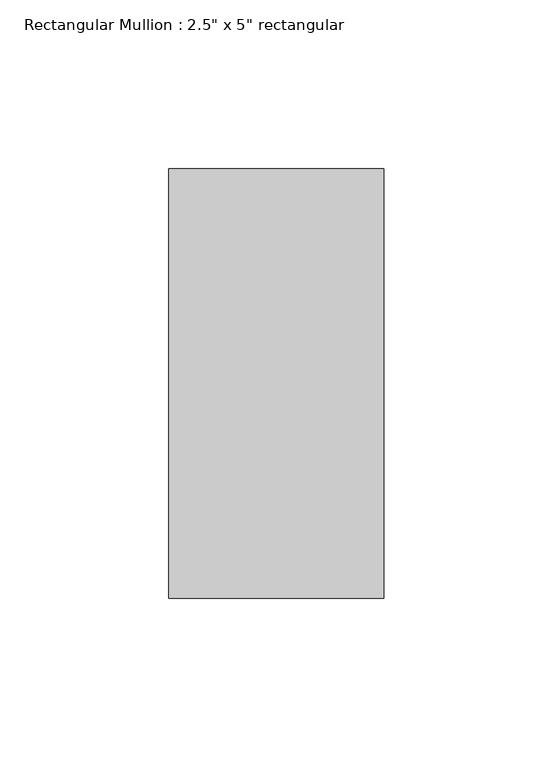
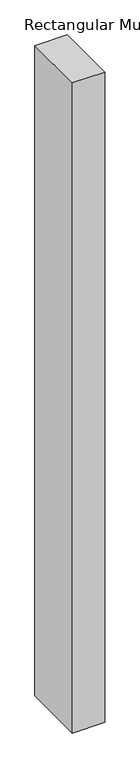
"""IFC4 building model written with IfcOpenShell, lengths in millimetres: member geometry."""

from ifc_helpers import new_model, si_unit, frame, origin, place, context, project, spatial, polyline, outline, extrude, source, transform, mapped, element, save


def member_d1dfe9dc(model_context):
    return source(origin(), model_context, "Body", "SweptSolid", [
        extrude(outline(polyline([(0.0, 63.5), (0.0, -63.5), (-63.5, -63.5), (-63.5, 63.5), (0.0, 63.5)])), frame((0.0, 0.0, -1341.7662723), z_axis=(0.0, 0.0, 1.0), x_axis=(1.0, 0.0, 0.0)), (0.0, 0.0, 1.0), 1341.7662723),
    ])


if __name__ == "__main__":
    model = new_model("IFC4")
    model_context = context("Model", 3, world=origin())
    ifc_project = project(units=[si_unit("LENGTHUNIT", "METRE", prefix="MILLI")], contexts=[model_context])
    site = spatial("IfcSite", under=ifc_project)
    building = spatial("IfcBuilding", under=site)
    placement = place(None, origin())
    member_shape = member_d1dfe9dc(model_context)
    element("IfcMember", 1, ObjectType="Rectangular Mullion : 2.5\" x 5\" rectangular", at=placement, inside=building, context=model_context, shape_type="MappedRepresentation", body=[
        mapped(member_shape, transform((0.0, 0.0, 0.0), x_axis=(1.0, 0.0, 0.0), y_axis=(0.0, 1.0, 0.0), z_axis=(0.0, 0.0, 1.0))),
    ])
    save(model, "model.ifc")

# Revit data of these elements
# Type "Rectangular Mullion : 2.5\" x 5\" rectangular"
#   built-in parameter 1007304 = 0.416667 (stored number, unit not read)
#   built-in parameter 1007301 = 0.104167 (stored number, unit not read)
#   built-in parameter 1007300 = 0.104167 (stored number, unit not read)
# Element 1 (IfcMember, "Rectangular Mullion : 2.5\" x 5\" rectangular")
#   Materials on its faces: "Aluminum"
# Materials
#   "Aluminum": class "Metal", colour RGB 247 247 247, transparency 0, Description = "Aluminum 6061", Cost = 0
